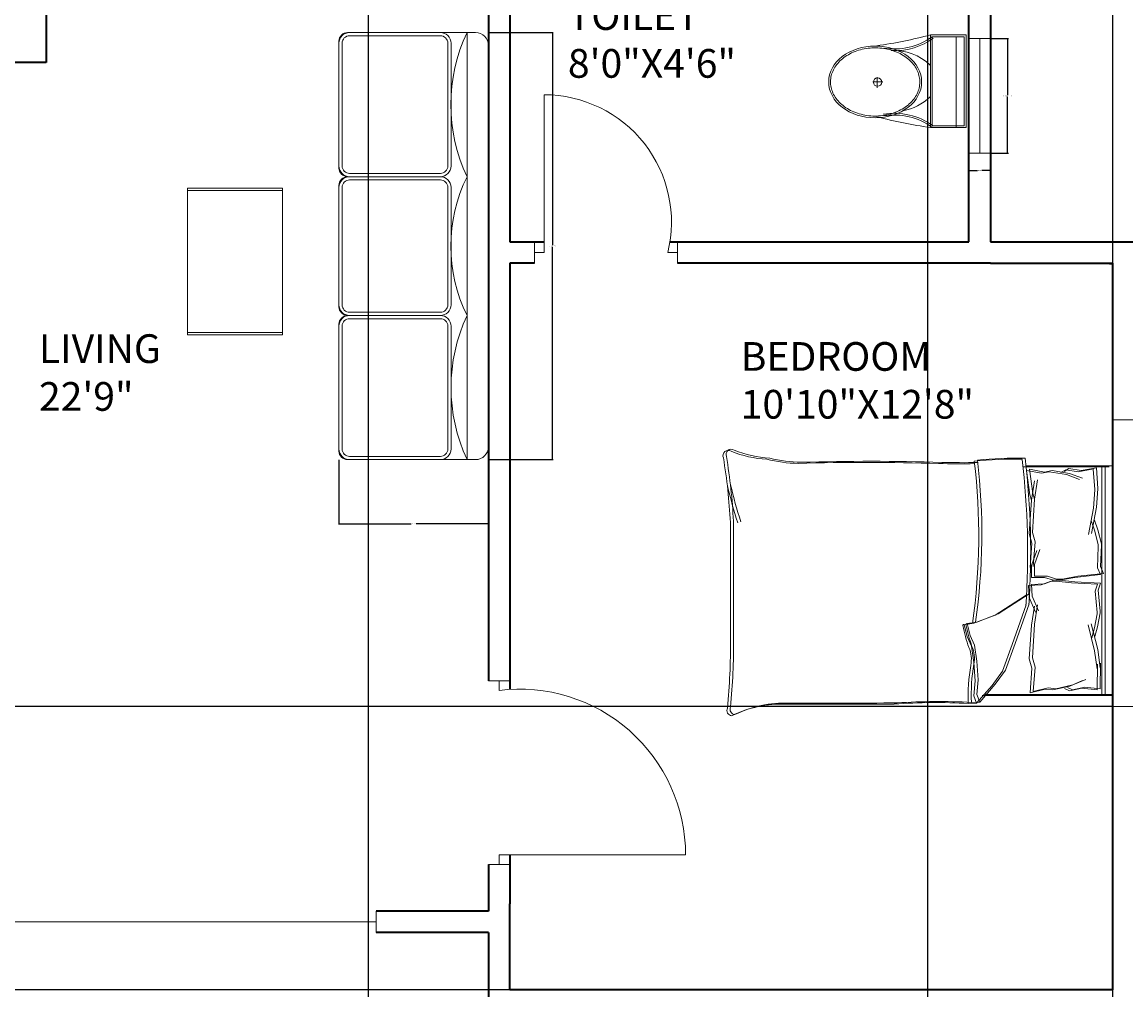
# Model space of a CAD drawing. Units: inches. Extents: x 1854 to 2495, y 1460 to 2772.
# Tile 4 of 12: x 2144 to 2375, y 1644 to 1847. Entities that reach past the tile are written whole.
import ezdxf

# ---------------------------------------------------------------- set-up
doc = ezdxf.new("R2010")
doc.units = ezdxf.units.IN
for name, color, linetype, lineweight in [('A-ANNO-DIMS', 2, 'Continuous', 18), ('A-AREA-IDEN', 7, 'Continuous', 18), ('A-DOOR', 3, 'Continuous', 18), ('A-FLOR-FIXT', 9, 'Continuous', 18), ('A-FURN', 8, 'Continuous', 13), ('A-GLAZ', 4, 'Continuous', 18), ('A-WALL', 7, 'Continuous', 35)]:
    doc.layers.add(name, color=color, linetype=linetype, lineweight=lineweight)
doc.styles.get("Standard").update_dxf_attribs({"font": 'arial.ttf'})
doc.dimstyles.get("Standard").update_dxf_attribs({"dimtxt": 0.18, "dimasz": 0.18, "dimexe": 0.18, "dimexo": 0.0625, "dimgap": 0.09, "dimtad": 0, "dimtih": 1, "dimtoh": 1, "dimdec": 4, "dimzin": 0, "dimdsep": 46, "dimtxsty": 'Standard', "dimcen": 0.09, "dimadec": 0, "dimazin": 0, "dimtfac": 1, "dimtdec": 4, "dimtofl": 0, "dimtmove": 0, "dimatfit": 3, "dimfxl": 1, "dimtolj": 1, "dimtzin": 0, "dimarcsym": 0})

# ---------------------------------------------------------------- blocks, each defined once
blk = doc.blocks.new('A$C31115884')
for p, q in [((283.1, 497.7), (223.4, 497.7)), ((257.5, 466.4), (257.5, 523.2)), ((0, 200), (0, 0)), ((520, 200), (0, 200)), ((10, 190), (10, 10)), ((510, 190), (10, 190)), ((510, 10), (510, 190)), ((520, 0), (520, 200)), ((510, 54.5), (0, 54.5)), ((10, 10), (510, 10)), ((0, 0), (520, 0))]:
    blk.add_line(p, q)
blk.add_circle((255.6, 496.4), 23.6)
for centre, radius, start, end in [((2777.7, -204.6), 2807, 165.4549, 171.71327), ((3237, 905), 2807, 188.28673, 194.5451), ((-294.5, 403.3), 364.7, 324.20913, 9.34987), ((-294.5, 403.3), 374.7, 324.20913, 9.34987), ((805.8, 403.3), 364.7, 170.65013, 215.79087), ((139.5, 406.2), 293.5, 315.84364, 2.65635), ((805.8, 403.3), 374.7, 179.20365, 215.79087), ((383.6, 406.2), 293.5, 190.27735, 224.15636)]:
    blk.add_arc(centre, radius, start, end)
blk.add_ellipse((256.2, 509.9), major_axis=(0, -260.7), ratio=0.772727)
blk.add_open_spline([(256.2, 259.2), (263.1, 259.2), (270, 259.7), (287.8, 262.3), (298.7, 265.1), (319.9, 273.1), (330.2, 278.4), (350.1, 291.1), (359.7, 298.7), (377.7, 315.9), (386.2, 325.5), (401.7, 346.6), (408.8, 358.1), (421.3, 382.5), (426.8, 395.5), (435.9, 422.4), (439.5, 436.4), (444.8, 465.1), (446.5, 479.7), (447.9, 509.2), (447.6, 524), (445, 553.3), (442.7, 567.8), (436.3, 596), (432.1, 609.7), (421.9, 636), (416, 648.6), (402.5, 672.1), (395, 683), (378.6, 703), (369.8, 712.1), (351.1, 728), (341.3, 734.8), (320.9, 746.2), (310.4, 750.7), (288.9, 757.3), (278, 759.4), (256, 761), (245, 760.6), (223.1, 757.2), (212.3, 754.3), (191.1, 746.1), (180.8, 740.7), (160.9, 727.8), (151.4, 720.1), (133.5, 702.7), (125.1, 693), (109.6, 671.7), (102.6, 660.2), (90.2, 635.7), (84.9, 622.7), (76, 595.6), (72.4, 581.6), (67.2, 552.9), (65.6, 538.2), (64.4, 508.8), (64.8, 494), (67.5, 464.7), (69.9, 450.2), (76.6, 422), (80.8, 408.3), (91.1, 382.2), (97.2, 369.7), (110.8, 346.3), (118.4, 335.4), (134.8, 315.6), (143.7, 306.7), (162.4, 290.9), (172.3, 284.2), (192.8, 273), (203.3, 268.6), (224.8, 262.2), (235.8, 260.2), (249.9, 259.3), (253, 259.2), (256.2, 259.2)], degree=3, knots=[0, 0, 0, 0, 0.110105, 0.110105, 0.285049, 0.285049, 0.459994, 0.459994, 0.634938, 0.634938, 0.809882, 0.809882, 0.984827, 0.984827, 1.159771, 1.159771, 1.334715, 1.334715, 1.50966, 1.50966, 1.684604, 1.684604, 1.859549, 1.859549, 2.034493, 2.034493, 2.209437, 2.209437, 2.384382, 2.384382, 2.559326, 2.559326, 2.73427, 2.73427, 2.909215, 2.909215, 3.084159, 3.084159, 3.259103, 3.259103, 3.434048, 3.434048, 3.608992, 3.608992, 3.783936, 3.783936, 3.958881, 3.958881, 4.133825, 4.133825, 4.30877, 4.30877, 4.483714, 4.483714, 4.658658, 4.658658, 4.833603, 4.833603, 5.008547, 5.008547, 5.183491, 5.183491, 5.358436, 5.358436, 5.53338, 5.53338, 5.708324, 5.708324, 5.883269, 5.883269, 6.058213, 6.058213, 6.233158, 6.233158, 6.283185, 6.283185, 6.283185, 6.283185])
blk = doc.blocks.new('BED-DOUBLE')
for p, q in [((30.13, 53.18), (28.39, 53.1, 3.87)), ((30.13, 53.18), (28.39, 53.1, 3.87)), ((0, 51.27), (0, 51.49)), ((0, 51.49), (0.64, 51.49)), ((0, 51.27), (26.61, 51.27)), ((0, 51.27), (26.61, 51.27)), ((0, 51.27), (0, 3.48)), ((0.64, 51.49), (27.25, 51.49)), ((0.64, 51.49), (27.25, 51.49)), ((1.53, 3.48), (1.53, 51.27)), ((1.53, 3.48), (1.53, 51.27)), ((2.17, 3.7), (2.17, 51.49)), ((2.17, 3.7), (2.17, 51.49)), ((17.21, 50.93), (14.07, 50.15)), ((17.21, 50.93), (14.07, 50.15)), ((16.81, 45.8), (17.21, 50.93)), ((16.81, 45.79), (17.21, 50.93)), ((27.75, 52.87), (24.5, 49.16)), ((27.75, 52.87), (24.5, 49.16)), ((28.39, 53.1), (25.14, 49.39)), ((28.39, 53.1), (25.14, 49.39)), ((29.49, 52.95), (27.75, 52.87, 3.87)), ((29.49, 52.95), (27.75, 52.87, 3.87)), ((28.37, 51.33), (27.75, 52.87)), ((28.37, 51.33), (27.75, 52.87)), ((28.06, 48.23), (28.37, 51.33)), ((28.06, 48.23), (28.37, 51.33)), ((29, 51.56), (28.39, 53.1)), ((29, 51.56), (28.39, 53.1)), ((28.7, 48.46), (29, 51.56)), ((28.7, 48.46), (29, 51.56)), ((2.56, 50.11), (2.46, 44.71)), ((2.56, 50.11), (2.46, 44.71)), ((2.56, 50.11), (5.77, 49.73)), ((2.56, 50.11), (5.77, 49.73)), ((3.2, 50.34), (3.1, 44.94)), ((3.2, 50.34), (3.1, 44.94)), ((3.2, 50.34), (6.41, 49.96)), ((3.2, 50.34), (6.41, 49.96)), ((8.26, 49.31), (5.58, 48.13)), ((8.26, 49.31), (5.58, 48.13)), ((5.77, 49.73), (8.34, 50.33)), ((5.77, 49.73), (8.34, 50.33)), ((8.9, 49.54), (6.22, 48.36)), ((8.9, 49.54), (6.22, 48.36)), ((6.41, 49.96), (8.98, 50.56)), ((6.41, 49.96), (8.98, 50.56)), ((11.83, 50.11), (8.26, 49.31)), ((11.83, 50.11), (8.26, 49.31)), ((8.34, 50.33), (9.38, 49.81)), ((8.34, 50.33), (9.38, 49.81)), ((12.47, 50.34), (8.9, 49.54)), ((12.47, 50.34), (8.9, 49.54)), ((8.98, 50.56), (10.02, 50.04)), ((8.98, 50.56), (10.02, 50.04)), ((13.43, 49.92), (11.83, 50.11)), ((13.43, 49.92), (11.83, 50.11)), ((14.07, 50.15), (12.47, 50.34)), ((14.07, 50.15), (12.47, 50.34)), ((16.57, 50.7), (13.43, 49.92)), ((16.57, 50.7), (13.43, 49.92)), ((16.17, 45.57), (16.57, 50.7)), ((16.17, 45.57), (16.57, 50.7)), ((24.5, 49.16), (22.33, 46.22)), ((24.5, 49.16), (22.33, 46.22)), ((25.14, 49.39), (22.97, 46.45)), ((25.14, 49.39), (22.97, 46.45)), ((22.33, 46.22), (20.32, 40.64)), ((22.33, 46.22), (20.32, 40.64)), ((22.97, 46.45), (20.96, 40.87)), ((22.97, 46.45), (20.96, 40.87)), ((28.37, 44.36), (28.06, 48.23)), ((28.37, 44.36), (28.06, 48.23)), ((29, 44.59), (28.7, 48.46)), ((29, 44.59), (28.7, 48.46)), ((2.46, 44.71), (2.54, 45.71)), ((2.46, 44.71), (2.54, 45.71)), ((2.54, 45.71), (3.07, 41.91)), ((2.54, 45.71), (3.07, 41.91)), ((3.1, 44.94), (3.18, 45.94)), ((3.1, 44.94), (3.18, 45.94)), ((3.18, 45.94), (3.71, 42.14)), ((3.18, 45.94), (3.71, 42.14)), ((16.73, 43.61), (16.17, 45.57)), ((16.73, 43.61), (16.17, 45.57)), ((17.37, 43.83), (16.81, 45.8)), ((17.37, 43.83), (16.81, 45.79)), ((28.83, 40.95), (28.37, 44.36)), ((28.83, 40.95), (28.37, 44.36)), ((29.47, 41.18), (29, 44.59)), ((29.47, 41.18), (29, 44.59)), ((3.07, 41.91), (4.42, 36.5)), ((3.07, 41.91), (4.42, 36.5)), ((3.71, 42.14), (5.06, 36.72)), ((3.71, 42.14), (5.06, 36.72)), ((16.3, 36.6), (16.73, 43.61)), ((16.3, 36.6), (16.73, 43.61)), ((16.93, 36.82), (17.37, 43.83)), ((16.93, 36.82), (17.37, 43.83)), ((4.31, 39.43), (3.72, 37.36)), ((4.31, 39.43), (3.72, 37.36)), ((20.32, 40.64), (17.38, 32.31)), ((20.32, 40.64), (17.38, 32.31)), ((20.96, 40.87), (18.02, 32.53)), ((20.96, 40.87), (18.02, 32.53)), ((29.76, 38.94), (28.83, 40.95)), ((29.76, 38.94), (28.83, 40.95)), ((30.4, 39.17), (29.47, 41.18)), ((30.4, 39.17), (29.47, 41.18)), ((79.25, 15.06), (79.25, 39.68)), ((79.25, 15.06), (79.25, 39.68)), ((79.88, 15.29), (79.88, 39.91)), ((79.88, 15.29), (79.88, 39.91)), ((3.08, 37.14), (2.54, 34.2)), ((3.08, 37.14), (2.54, 34.2)), ((3.67, 39.2), (3.08, 37.14)), ((3.67, 39.2), (3.08, 37.14)), ((3.72, 37.36), (3.18, 34.43)), ((3.72, 37.36), (3.18, 34.43)), ((30.38, 36.46), (29.76, 38.94)), ((30.38, 36.46), (29.76, 38.94)), ((31.02, 36.69), (30.4, 39.17)), ((31.02, 36.69), (30.4, 39.17)), ((15.63, 32.56), (16.3, 36.6)), ((15.63, 32.56), (16.3, 36.6)), ((16.27, 32.79), (16.93, 36.82)), ((16.27, 32.79), (16.93, 36.82)), ((18.02, 30.49), (24.52, 34.68)), ((18.02, 30.49), (24.52, 34.68)), ((23.88, 34.45), (28.37, 36.15)), ((23.88, 34.45), (28.37, 36.15)), ((24.52, 34.68), (29, 36.38)), ((24.52, 34.68), (29, 36.38)), ((28.37, 36.15), (30.38, 36.46)), ((28.37, 36.15), (30.38, 36.46)), ((29, 36.38), (31.02, 36.69)), ((29, 36.38), (31.02, 36.69)), ((2.54, 34.2), (2.56, 33.88)), ((2.54, 34.2), (2.56, 33.88)), ((2.56, 33.88), (2.98, 29.46)), ((2.56, 33.88), (2.98, 29.46)), ((3.18, 34.43), (3.2, 34.11)), ((3.18, 34.43), (3.2, 34.11)), ((3.2, 34.11), (3.62, 29.68)), ((3.2, 34.11), (3.62, 29.68)), ((16.74, 30.75), (15.45, 33.82)), ((16.74, 30.75), (15.45, 33.82)), ((17.38, 30.98), (16.09, 34.05)), ((17.38, 30.98), (16.09, 34.05)), ((17.38, 30.26), (23.88, 34.45)), ((17.38, 30.26), (23.88, 34.45)), ((16.89, 28.3), (16.74, 30.75)), ((16.89, 28.3), (16.74, 30.75)), ((17.53, 28.53), (17.38, 30.98)), ((17.53, 28.53), (17.38, 30.98)), ((2.98, 29.46), (2.49, 27.98)), ((2.98, 29.46), (2.49, 27.98)), ((2.49, 27.98), (7.87, 27.73)), ((2.49, 27.98), (7.87, 27.73)), ((3.62, 29.68), (3.13, 28.21)), ((3.62, 29.68), (3.13, 28.21)), ((3.13, 28.21), (8.51, 27.96)), ((3.13, 28.21), (8.51, 27.96)), ((7.87, 27.73), (11.08, 27.36)), ((7.87, 27.73), (11.08, 27.35)), ((8.51, 27.96), (11.72, 27.58)), ((8.51, 27.96), (11.72, 27.58)), ((12.38, 27.44), (14.22, 28.13)), ((12.38, 27.44), (14.22, 28.13)), ((13.02, 27.66), (14.86, 28.36)), ((13.02, 27.66), (14.86, 28.36)), ((14.22, 28.13), (16.89, 28.3)), ((14.22, 28.13), (16.89, 28.3)), ((14.86, 28.36), (17.53, 28.53)), ((14.86, 28.36), (17.53, 28.53)), ((1.87, 25.98), (7.22, 26.56)), ((1.87, 25.98), (7.22, 26.56)), ((2.45, 24.54), (1.87, 25.98)), ((2.45, 24.54), (1.87, 25.98)), ((2.51, 26.21), (7.86, 26.79)), ((2.51, 26.21), (7.86, 26.79)), ((3.09, 24.77), (2.51, 26.21)), ((3.09, 24.77), (2.51, 26.21)), ((7.22, 26.56), (10.4, 27.14)), ((7.22, 26.56), (10.4, 27.14)), ((7.86, 26.79), (11.04, 27.37)), ((7.86, 26.79), (11.04, 27.37)), ((10.4, 27.14), (11.7, 27.14)), ((10.4, 27.14), (11.7, 27.14)), ((11.04, 27.37), (12.34, 27.37)), ((11.04, 27.37), (12.34, 27.37)), ((11.08, 27.36), (12.38, 27.44)), ((11.08, 27.35), (12.38, 27.44)), ((11.7, 27.14), (13.58, 26.56)), ((11.7, 27.14), (13.58, 26.56)), ((11.72, 27.58), (13.02, 27.66)), ((11.72, 27.58), (13.02, 27.66)), ((12.34, 27.37), (14.22, 26.79)), ((12.34, 27.37), (14.22, 26.79)), ((13.58, 26.56), (16.26, 26.56)), ((13.58, 26.56), (16.26, 26.56)), ((14.22, 26.79), (16.9, 26.79)), ((14.22, 26.79), (16.9, 26.79)), ((16.26, 26.56), (16.26, 24.1)), ((16.26, 26.56), (16.26, 24.1)), ((16.9, 26.79), (16.9, 24.33)), ((16.9, 26.79), (16.9, 24.33)), ((2.3, 20.09), (2.45, 24.54)), ((2.3, 20.09), (2.45, 24.54)), ((2.94, 20.32), (3.09, 24.77)), ((2.94, 20.32), (3.09, 24.77)), ((16.26, 24.1), (15.17, 20.96)), ((16.26, 24.1), (15.17, 20.96)), ((16.9, 24.33), (15.81, 21.19)), ((16.9, 24.33), (15.81, 21.19)), ((16.17, 19.38), (16.57, 24.52)), ((16.17, 19.38), (16.57, 24.52)), ((16.81, 19.61), (17.21, 24.74)), ((16.81, 19.61), (17.21, 24.74)), ((2.3, 19.77), (2.3, 20.09)), ((2.3, 19.77), (2.3, 20.09)), ((3.03, 16.88), (2.3, 19.77)), ((3.03, 16.88), (2.3, 19.77)), ((2.94, 20), (2.94, 20.32)), ((2.94, 20), (2.94, 20.32)), ((3.67, 17.11), (2.94, 20)), ((3.67, 17.11), (2.94, 20)), ((16.73, 17.42), (16.17, 19.38)), ((16.73, 17.42), (16.17, 19.38)), ((17.37, 17.65), (16.81, 19.61)), ((17.37, 17.65), (16.81, 19.61)), ((3.75, 14.86), (3.03, 16.88)), ((3.75, 14.85), (3.03, 16.88)), ((3.32, 12.11), (4.33, 17.6)), ((3.32, 12.11), (4.33, 17.6)), ((4.39, 15.08), (3.67, 17.11)), ((4.39, 15.08), (3.67, 17.11)), ((3.96, 12.34), (4.97, 17.83)), ((3.96, 12.34), (4.97, 17.83)), ((16.3, 10.41), (16.73, 17.42)), ((16.3, 10.41), (16.73, 17.42)), ((16.93, 10.64), (17.37, 17.65)), ((16.93, 10.64), (17.37, 17.65)), ((3.03, 8.29), (3.32, 12.11)), ((3.03, 8.28), (3.32, 12.11)), ((3.67, 8.51), (3.96, 12.34)), ((3.67, 8.51), (3.96, 12.34)), ((15.63, 6.38), (16.3, 10.41)), ((15.63, 6.38), (16.3, 10.41)), ((16.27, 6.61), (16.93, 10.64)), ((16.27, 6.61), (16.93, 10.64)), ((16.3, 10.41), (16.62, 9.28)), ((16.3, 10.41), (16.62, 9.28)), ((16.62, 9.28), (17.34, 4.18)), ((16.62, 9.28), (17.34, 4.18)), ((16.93, 10.64), (17.26, 9.51)), ((16.93, 10.64), (17.26, 9.51)), ((17.26, 9.51), (17.98, 4.41)), ((17.26, 9.51), (17.98, 4.41)), ((3.01, 8.18), (3.03, 8.29)), ((3.01, 8.18), (3.03, 8.28)), ((3.34, 3.9), (3.01, 8.18)), ((3.34, 3.9), (3.01, 8.18)), ((3.65, 8.41), (3.67, 8.51)), ((3.65, 8.41), (3.67, 8.51)), ((3.98, 4.13), (3.65, 8.41)), ((3.98, 4.13), (3.65, 8.41)), ((3.96, 4.12), (7.14, 4.7)), ((3.96, 4.12), (7.14, 4.7)), ((8.96, 5.05), (6.21, 6.06)), ((8.96, 5.05), (6.21, 6.06)), ((9.59, 5.28), (6.85, 6.29)), ((9.59, 5.28), (6.85, 6.29)), ((7.14, 4.7), (9.74, 4.27)), ((7.14, 4.7), (9.74, 4.27)), ((12.57, 4.47), (8.96, 5.05)), ((12.57, 4.47), (8.96, 5.05)), ((9.1, 4.04), (10.11, 4.62)), ((13.21, 4.7), (9.59, 5.28)), ((13.21, 4.7), (9.59, 5.28)), ((9.74, 4.27), (10.75, 4.85)), ((9.74, 4.27), (10.75, 4.85)), ((14.16, 4.76), (12.57, 4.47)), ((14.16, 4.76), (12.57, 4.47)), ((14.8, 4.99), (13.21, 4.7)), ((14.8, 4.99), (13.21, 4.7)), ((17.34, 4.18), (14.16, 4.76)), ((17.34, 4.18), (14.16, 4.76)), ((17.98, 4.41), (14.8, 4.99)), ((17.98, 4.41), (14.8, 4.99)), ((18.11, 3.48), (0, 3.48)), ((18.11, 3.48), (0, 3.48)), ((18.75, 3.7), (0.64, 3.7)), ((18.75, 3.7), (0.64, 3.7)), ((3.32, 3.89), (6.5, 4.47)), ((3.32, 3.89), (6.5, 4.47)), ((6.5, 4.47), (9.1, 4.04)), ((6.5, 4.47), (9.1, 4.04)), ((9.1, 4.04), (10.11, 4.62))]:
    blk.add_line(p, q)
for centre, radius, start, end in [((68.67, 76.16), 23.07, 267.4714, 296.4681), ((68.67, 76.16), 23.07, 267.4714, 296.4681), ((69.31, 76.39), 23.07, 267.4714, 296.4681), ((69.31, 76.39), 23.07, 267.4714, 296.4681), ((78.87, 54.41), 1.1, 332.6588, 86.02), ((78.87, 54.41), 1.1, 332.6588, 86.02), ((79.51, 54.64), 1.1, 332.6588, 86.02), ((79.51, 54.64), 1.1, 332.6588, 86.02), ((-6.02, 51.56), 36.18, 349.8763, 2.5657), ((-6.02, 51.56), 36.18, 349.8763, 2.5657), ((36.95, 182.49), 129.5, 266.9791, 273.8365), ((36.95, 182.49), 129.5, 266.9791, 273.8365), ((67.82, -4508.74), 4561.86, 90.00217, 90.28689), ((67.82, -4508.74), 4561.86, 90.00217, 90.28689), ((68.46, -4508.51), 4561.86, 90.00217, 90.28689), ((68.46, -4508.52), 4561.86, 90.00217, 90.28689), ((212.28, 41.15), 133.04, 174.4998, 180.6351), ((212.28, 41.15), 133.04, 174.4998, 180.6351), ((212.92, 41.38), 133.04, 174.4998, 180.6351), ((212.92, 41.38), 133.04, 174.4998, 180.6351), ((-6.66, 51.33), 36.18, 349.8763, 2.5657), ((-6.66, 51.33), 36.18, 349.8763, 2.5657), ((36.32, 182.27), 129.5, 266.9791, 273.8365), ((36.32, 182.27), 129.5, 266.9791, 273.8365), ((35.07, 43.74), 6.22, 168.6608, 203.7384), ((35.07, 43.74), 6.22, 168.6608, 203.7384), ((35.71, 43.97), 6.22, 168.6608, 203.7384), ((35.71, 43.97), 6.22, 168.6608, 203.7384), ((1.48, 31.15), 29.65, 10.6617, 19.8806), ((1.48, 31.15), 29.65, 10.6617, 19.8806), ((2.12, 31.38), 29.65, 10.6617, 19.8806), ((2.12, 31.38), 29.65, 10.6617, 19.8806), ((156.32, 17.76), 129.02, 171.7845, 186.9006), ((156.32, 17.76), 129.02, 171.7845, 186.9006), ((156.96, 17.98), 129.02, 171.7845, 186.9006), ((156.96, 17.98), 129.02, 171.7845, 186.9006), ((30.44, 36.64), 0.185, 250.2464, 1.1377), ((30.44, 36.64), 0.185, 250.2464, 1.1377), ((31.08, 36.86), 0.185, 250.2464, 1.1377), ((31.08, 36.86), 0.185, 250.2464, 1.1377), ((182.05, 21.36), 164.97, 176.0865, 186.7821), ((182.05, 21.36), 164.97, 176.0865, 186.7821), ((182.69, 21.59), 164.97, 176.0865, 186.7821), ((182.69, 21.59), 164.97, 176.0865, 186.7821), ((-23.71, -17.22), 106.46, 13.3832, 17.7053), ((-23.71, -17.22), 106.46, 13.3832, 17.7053), ((-23.07, -16.99), 106.46, 13.3832, 17.7053), ((-23.07, -16.99), 106.46, 13.3832, 17.7053), ((200.84, 21.43), 121.76, 182.9958, 189.4091), ((200.84, 21.43), 121.76, 182.9958, 189.4091), ((201.48, 21.66), 121.76, 182.9958, 189.4091), ((201.48, 21.66), 121.76, 182.9958, 189.4091), ((20.74, 85.39), 83.31, 268.7218, 275.604), ((20.74, 85.39), 83.31, 268.7218, 275.604), ((31.17, -167.31), 170.11, 88.4762, 91.0082), ((31.17, -167.31), 170.11, 88.4762, 91.0082), ((31.81, -167.08), 170.11, 88.4762, 91.0082), ((31.81, -167.08), 170.11, 88.4762, 91.0082), ((50.61, 484.82), 482.31, 268.2277, 271.7185), ((50.61, 484.82), 482.31, 268.2277, 271.7185), ((51.25, 485.05), 482.31, 268.2277, 271.7185), ((51.25, 485.05), 482.31, 268.2277, 271.7185), ((64.52, -26.9), 29.63, 76.0648, 88.9113), ((64.52, -26.9), 29.63, 76.0648, 88.9113), ((65.15, -26.67), 29.63, 76.0648, 88.9113), ((65.15, -26.67), 29.63, 76.0648, 88.9113), ((20.1, 85.16), 83.31, 268.7218, 275.604), ((20.1, 85.16), 83.31, 268.7218, 275.604), ((70.28, -21.66), 23.56, 67.9751, 86.652), ((70.28, -21.66), 23.56, 67.9751, 86.652), ((70.92, -21.43), 23.56, 67.9751, 86.652), ((70.92, -21.43), 23.56, 67.9751, 86.652), ((79.72, 1.09), 1.09, 236.1736, 23.4781), ((79.72, 1.09), 1.09, 236.1736, 23.4781), ((80.36, 1.32), 1.09, 236.1736, 23.4781), ((80.36, 1.32), 1.09, 236.1736, 23.4781)]:
    blk.add_arc(centre, radius, start, end)
blk = doc.blocks.new('TABLE-COFFEE')
blk.add_lwpolyline([(0, 30.16), (19.85, 30.16), (19.85, 0), (0, 0)], close=True)
blk = doc.blocks.new('WINDOW-60IN')
for p, q in [((0, 9), (0, 0)), ((60, 4.5), (60, 9)), ((60, 9), (60, 0)), ((0, 0), (0, 4.5)), ((0, 4.5), (60, 4.5))]:
    blk.add_line(p, q)
blk = doc.blocks.new('DOOR-39IN-SWING')
blk.add_line((39, 0), (0, 0))
blk.add_arc((34.67, 0), 34.66, 82.8159, 180)
blk = doc.blocks.new('WINDOW-VENT-24IN-INTERIOR')
for p, q in [((0, 24), (4.5, 24)), ((2.25, 24), (2.25, 0)), ((0, 0), (4.5, 0))]:
    blk.add_line(p, q)
blk = doc.blocks.new('SOFA-3-SEAT')
for points in [[(2.23, 59.19), (21.22, 59.19, 0.414214), (23.45, 61.43), (23.45, 87.12, 0.414214), (21.22, 89.35), (2.23, 89.35, 0.414214), (0, 87.12), (0, 61.43, 0.414214)], [(2.23, 59.19), (21.22, 59.19, -0.414214), (23.45, 56.96), (23.45, 32.39, -0.414214), (21.22, 30.16), (2.23, 30.16, -0.414214), (0, 32.39), (0, 56.96, -0.414214)], [(2.23, 0), (21.22, 0, 0.414214), (23.45, 2.23), (23.45, 27.92, 0.414214), (21.22, 30.16), (2.23, 30.16, 0.414214), (0, 27.92), (0, 2.23, 0.414214)]]:
    blk.add_lwpolyline(points, format="xyb", close=True)
at = {"ltscale": 0.03}
blk.add_lwpolyline([(0, 28.35), (0, 1.79, 0.414214), (1.79, 0), (28.59, 0, 0.414214), (31.27, 2.68), (31.27, 86.67, 0.414214), (28.59, 89.35), (1.79, 89.35, 0.414214), (0, 87.56), (0, 61, 0.414214), (1.79, 59.22, -1), (1.79, 59.17, 0.414214), (0, 57.38), (0, 31.96, 0.414214), (1.79, 30.18, -1), (1.79, 30.13, 0.414214)], format="xyb", close=True, dxfattribs=at)
blk.add_lwpolyline([(26.8, 0), (26.8, 89.35)])
for centre, radius, start, end in [((58.64, 74.27), 35.22, 154.6538, 205.3462), ((56.4, 44.67), 32.97, 153.869, 206.131), ((59.01, 15.08), 35.56, 154.9106, 205.0894)]:
    blk.add_arc(centre, radius, start, end)
blk = doc.blocks.new('*D37')
at = {"layer": 'A-ANNO-DIMS', "color": 0, "lineweight": -2, "transparency": 16777216}
for p, q in [((2346.54, 1843.06), (2350.26, 1843.06)), ((2350.08, 1842.88), (2350.08, 1831.24)), ((2350.08, 1819.24), (2350.08, 1830.88)), ((2346.54, 1819.06), (2350.26, 1819.06))]:
    blk.add_line(p, q, dxfattribs=at)
at = {"layer": 'A-ANNO-DIMS', "color": 0, "transparency": 16777216}
for points in [[(2350.05, 1842.88), (2350.11, 1842.88), (2350.08, 1843.06)], [(2350.05, 1819.24), (2350.11, 1819.24), (2350.08, 1819.06)]]:
    blk.add_solid(points, dxfattribs=at)
at = {"layer": 'Defpoints', "color": 0, "transparency": 16777216}
for p in [(2346.48, 1843.06), (2350.08, 1843.06), (2346.48, 1819.06)]:
    blk.add_point(p, dxfattribs=at)
at = {"layer": 'A-ANNO-DIMS', "color": 0, "transparency": 16777216, "insert": (2350.08, 1831.06), "char_height": 0.18, "attachment_point": 5}
blk.add_mtext('\\A1;INT. VENT 24 TYP.', dxfattribs=at)
blk = doc.blocks.new('*D38')
at = {"layer": 'A-ANNO-DIMS', "color": 0, "lineweight": -2, "transparency": 16777216}
for p, q in [((2341.98, 1819), (2341.98, 1815.28)), ((2346.48, 1819), (2346.48, 1815.28)), ((2342.16, 1815.46), (2343.77, 1815.46)), ((2346.3, 1815.46), (2344.69, 1815.46))]:
    blk.add_line(p, q, dxfattribs=at)
at = {"layer": 'A-ANNO-DIMS', "color": 0, "transparency": 16777216}
for points in [[(2342.16, 1815.49), (2342.16, 1815.43), (2341.98, 1815.46)], [(2346.3, 1815.49), (2346.3, 1815.43), (2346.48, 1815.46)]]:
    blk.add_solid(points, dxfattribs=at)
at = {"layer": 'Defpoints', "color": 0, "transparency": 16777216}
for p in [(2341.98, 1819.06), (2346.48, 1819.06), (2346.48, 1815.46)]:
    blk.add_point(p, dxfattribs=at)
at = {"layer": 'A-ANNO-DIMS', "color": 0, "transparency": 16777216, "insert": (2344.23, 1815.46), "char_height": 0.18, "attachment_point": 5}
blk.add_mtext('\\A1;5 TYP.', dxfattribs=at)
blk = doc.blocks.new('*D47')
at = {"layer": 'A-ANNO-DIMS', "color": 0, "lineweight": -2, "transparency": 16777216}
for p, q in [((2241.54, 1844.33), (2255.06, 1844.33)), ((2254.88, 1844.15), (2254.88, 1799.84)), ((2254.88, 1755.16), (2254.88, 1799.47)), ((2241.54, 1754.98), (2255.06, 1754.98))]:
    blk.add_line(p, q, dxfattribs=at)
at = {"layer": 'A-ANNO-DIMS', "color": 0, "transparency": 16777216}
for points in [[(2254.85, 1844.15), (2254.91, 1844.15), (2254.88, 1844.33)], [(2254.85, 1755.16), (2254.91, 1755.16), (2254.88, 1754.98)]]:
    blk.add_solid(points, dxfattribs=at)
at = {"layer": 'Defpoints', "color": 0, "transparency": 16777216}
for p in [(2241.48, 1844.33), (2254.88, 1844.33), (2241.48, 1754.98)]:
    blk.add_point(p, dxfattribs=at)
at = {"layer": 'A-ANNO-DIMS', "color": 0, "transparency": 16777216, "insert": (2254.88, 1799.66), "char_height": 0.18, "attachment_point": 5}
blk.add_mtext('\\A1;SOFA 89 TYP.', dxfattribs=at)
blk = doc.blocks.new('*D48')
at = {"layer": 'A-ANNO-DIMS', "color": 0, "lineweight": -2, "transparency": 16777216}
for p, q in [((2210.21, 1754.92), (2210.21, 1741.4)), ((2241.48, 1754.92), (2241.48, 1741.4)), ((2210.39, 1741.58), (2225.32, 1741.58)), ((2241.3, 1741.58), (2226.37, 1741.58))]:
    blk.add_line(p, q, dxfattribs=at)
at = {"layer": 'A-ANNO-DIMS', "color": 0, "transparency": 16777216}
for points in [[(2210.39, 1741.61), (2210.39, 1741.55), (2210.21, 1741.58)], [(2241.3, 1741.61), (2241.3, 1741.55), (2241.48, 1741.58)]]:
    blk.add_solid(points, dxfattribs=at)
at = {"layer": 'Defpoints', "color": 0, "transparency": 16777216}
for p in [(2210.21, 1754.98), (2241.48, 1754.98), (2241.48, 1741.58)]:
    blk.add_point(p, dxfattribs=at)
at = {"layer": 'A-ANNO-DIMS', "color": 0, "transparency": 16777216, "insert": (2225.85, 1741.58), "char_height": 0.18, "attachment_point": 5}
blk.add_mtext('\\A1;31 TYP.', dxfattribs=at)
blk = doc.blocks.new('*D50')
at = {"layer": 'A-ANNO-DIMS', "color": 0, "lineweight": -2, "transparency": 16777216}
for p, q in [((2381.04, 2272.04), (2418.21, 2272.04)), ((2418.03, 2271.86), (2418.03, 1933.48)), ((2418.03, 1594.72), (2418.03, 1933.11)), ((2119.04, 1594.54), (2418.21, 1594.54))]:
    blk.add_line(p, q, dxfattribs=at)
at = {"layer": 'A-ANNO-DIMS', "color": 0, "transparency": 16777216}
for points in [[(2418, 2271.86), (2418.06, 2271.86), (2418.03, 2272.04)], [(2418, 1594.72), (2418.06, 1594.72), (2418.03, 1594.54)]]:
    blk.add_solid(points, dxfattribs=at)
at = {"layer": 'Defpoints', "color": 0, "transparency": 16777216}
for p in [(2380.98, 2272.04), (2418.03, 2272.04), (2118.98, 1594.54)]:
    blk.add_point(p, dxfattribs=at)
at = {"layer": 'A-ANNO-DIMS', "color": 0, "transparency": 16777216, "insert": (2418.03, 1933.29), "char_height": 0.18, "attachment_point": 5}
blk.add_mtext('\\A1;677.5', dxfattribs=at)
blk = doc.blocks.new('*D64')
at = {"layer": 'A-ANNO-DIMS', "color": 0, "lineweight": -2, "transparency": 16777216}
for p, q in [((2333.32, 2262.98), (2333.32, 1503.44)), ((2371.98, 2262.98), (2371.98, 1503.44)), ((2333.5, 1503.62), (2352.26, 1503.62)), ((2371.8, 1503.62), (2353.05, 1503.62))]:
    blk.add_line(p, q, dxfattribs=at)
at = {"layer": 'A-ANNO-DIMS', "color": 0, "transparency": 16777216}
for points in [[(2333.5, 1503.65), (2333.5, 1503.59), (2333.32, 1503.62)], [(2371.8, 1503.65), (2371.8, 1503.59), (2371.98, 1503.62)]]:
    blk.add_solid(points, dxfattribs=at)
at = {"layer": 'Defpoints', "color": 0, "transparency": 16777216}
for p in [(2333.32, 2263.04), (2371.98, 2263.04), (2371.98, 1503.62)]:
    blk.add_point(p, dxfattribs=at)
at = {"layer": 'A-ANNO-DIMS', "color": 0, "transparency": 16777216, "insert": (2352.65, 1503.62), "char_height": 0.18, "attachment_point": 5}
blk.add_mtext('\\A1;38.66', dxfattribs=at)
blk = doc.blocks.new('*D66')
at = {"layer": 'A-ANNO-DIMS', "color": 0, "lineweight": -2, "transparency": 16777216}
for p, q in [((2371.92, 1703.31), (1940.75, 1703.31)), ((1940.93, 1703.13), (1940.93, 1673.86)), ((1940.93, 1644.22), (1940.93, 1673.5)), ((2371.92, 1644.04), (1940.75, 1644.04))]:
    blk.add_line(p, q, dxfattribs=at)
at = {"layer": 'A-ANNO-DIMS', "color": 0, "transparency": 16777216}
for points in [[(1940.9, 1703.13), (1940.96, 1703.13), (1940.93, 1703.31)], [(1940.9, 1644.22), (1940.96, 1644.22), (1940.93, 1644.04)]]:
    blk.add_solid(points, dxfattribs=at)
at = {"layer": 'Defpoints', "color": 0, "transparency": 16777216}
for p in [(1940.93, 1703.31), (2371.98, 1703.31), (2371.98, 1644.04)]:
    blk.add_point(p, dxfattribs=at)
at = {"layer": 'A-ANNO-DIMS', "color": 0, "transparency": 16777216, "insert": (1940.93, 1673.68), "char_height": 0.18, "attachment_point": 5}
blk.add_mtext('\\A1;59.27', dxfattribs=at)
blk = doc.blocks.new('*D73')
at = {"layer": 'A-ANNO-DIMS', "color": 0, "lineweight": -2, "transparency": 16777216}
for p, q in [((2131.08, 2220.98), (2131.08, 1503.44)), ((2216.32, 2220.98), (2216.32, 1503.44)), ((2131.26, 1503.62), (2173.31, 1503.62)), ((2216.14, 1503.62), (2174.1, 1503.62))]:
    blk.add_line(p, q, dxfattribs=at)
at = {"layer": 'A-ANNO-DIMS', "color": 0, "transparency": 16777216}
for points in [[(2131.26, 1503.65), (2131.26, 1503.59), (2131.08, 1503.62)], [(2216.14, 1503.65), (2216.14, 1503.59), (2216.32, 1503.62)]]:
    blk.add_solid(points, dxfattribs=at)
at = {"layer": 'Defpoints', "color": 0, "transparency": 16777216}
for p in [(2131.08, 2221.04), (2216.32, 2221.04), (2216.32, 1503.62)]:
    blk.add_point(p, dxfattribs=at)
at = {"layer": 'A-ANNO-DIMS', "color": 0, "transparency": 16777216, "insert": (2173.7, 1503.62), "char_height": 0.18, "attachment_point": 5}
blk.add_mtext('\\A1;85.25', dxfattribs=at)

msp = doc.modelspace()

# ---------------------------------------------------------------- linework, layer by layer
at = {"layer": 'A-DOOR'}
for p, q in [((2253.1289, 1798.3071), (2253.1289, 1831.3071)), ((2251.1289, 1800.5571), (2251.1289, 1796.0571)), ((2281.0007, 1800.5571), (2281.0007, 1796.0571)), ((2251.1289, 1796.0571), (2251.1289, 1798.3071)), ((2251.1289, 1798.3071), (2253.1289, 1798.3071)), ((2281.0007, 1798.3071), (2279.0007, 1798.3071)), ((2281.0007, 1796.0571), (2281.0007, 1798.3071)), ((2241.4824, 1708.6844), (2245.9824, 1708.6844)), ((2245.9824, 1708.6844), (2243.7324, 1708.6844)), ((2243.7324, 1708.6844), (2243.7324, 1706.6844)), ((2243.7324, 1670.2917), (2243.7324, 1672.2917)), ((2241.4824, 1670.2917), (2245.9824, 1670.2917)), ((2245.9824, 1670.2917), (2243.7324, 1670.2917))]:
    msp.add_line(p, q, dxfattribs=at)
msp.add_arc((2253.1289, 1804.6655), 26.6417, 346.192433, 90, dxfattribs=at)
at = {"layer": 'A-FURN'}
for points in [[(2212.444, 1814.8445), (2231.4306, 1814.8445, 0.41421356), (2232.9942, 1816.4081), (2232.9942, 1842.0959, 0.41421356), (2231.4306, 1843.6595), (2212.444, 1843.6595, 0.41421356), (2210.8804, 1842.0959), (2210.8804, 1816.4081, 0.41421356)], [(2212.444, 1813.5042), (2231.4306, 1813.5042, -0.41421356), (2232.9942, 1811.9406), (2232.9942, 1787.3696, -0.41421356), (2231.4306, 1785.806), (2212.444, 1785.806, -0.41421356), (2210.8804, 1787.3696), (2210.8804, 1811.9406, -0.41421356)], [(2212.444, 1755.6507), (2231.4306, 1755.6507, 0.41421356), (2232.9942, 1757.2143), (2232.9942, 1782.9022, 0.41421356), (2231.4306, 1784.4658), (2212.444, 1784.4658, 0.41421356), (2210.8804, 1782.9022), (2210.8804, 1757.2143, 0.41421356)]]:
    msp.add_lwpolyline(points, format="xyb", close=True, dxfattribs=at)
at = {"layer": 'A-GLAZ'}
for p, q in [((2346.4824, 1843.0598), (2344.2324, 1843.0598)), ((2344.2324, 1819.0598), (2341.9824, 1819.0598)), ((2218.0111, 1660.5449), (2218.0111, 1656.0449)), ((2218.0111, 1658.2949), (2140.0894, 1658.2949)), ((2218.0111, 1656.0449), (2218.0111, 1658.2949))]:
    msp.add_line(p, q, dxfattribs=at)
at = {"layer": 'A-WALL'}
for p, q in [((2148.9824, 1928.5287), (2148.9824, 1838.0449)), ((2241.4824, 1859.0571), (2241.4824, 1708.6844)), ((2245.9824, 1854.5571), (2245.9824, 1800.5571)), ((2245.9824, 1854.5571), (2245.9824, 1800.5571)), ((2341.9824, 1800.5571), (2341.9824, 1854.5571)), ((2346.4824, 1854.5571), (2346.4824, 1800.5571)), ((2148.9824, 1838.0449), (2139.9824, 1838.0449)), ((2245.9824, 1800.5571), (2253.1289, 1800.5571)), ((2279.4519, 1800.5571), (2341.9824, 1800.5571)), ((2346.4824, 1800.5571), (2380.9824, 1800.5571)), ((2371.9824, 1800.5571), (2371.9824, 1800.5449)), ((2371.9824, 1800.5571), (2371.9824, 1800.5449)), ((2251.1289, 1796.0571), (2245.9824, 1796.0571)), ((2245.9824, 1796.0571), (2245.9824, 1706.8938)), ((2346.4824, 1796.0571), (2281.0007, 1796.0571)), ((2346.4824, 1796.0571), (2371.9824, 1796.0571)), ((2371.391, 1796.0449), (2371.9824, 1796.0449)), ((2371.9824, 1796.0571), (2371.9824, 1662.0571)), ((2371.9824, 1796.0571), (2371.9824, 1644.0571)), ((2371.9824, 1796.0449), (2371.9824, 1644.0449)), ((2245.9824, 1672.2917), (2245.9824, 1662.0571)), ((2241.4824, 1670.2917), (2241.4824, 1662.0571)), ((2241.4824, 1660.5449), (2218.0111, 1660.5449)), ((2241.4824, 1662.0571), (2241.4824, 1660.5449)), ((2245.9824, 1644.0449), (2245.9824, 1662.0571)), ((2241.4824, 1656.0449), (2218.0111, 1656.0449)), ((2241.4824, 1656.0449), (2241.4824, 1644.0449)), ((2241.4824, 1644.0449), (2241.4824, 1635.0449)), ((2371.9824, 1644.0449), (2245.9824, 1644.0449))]:
    msp.add_line(p, q, dxfattribs=at)

# ---------------------------------------------------------------- block references
at = {"layer": 'A-DOOR', "extrusion": (0, 0, -1), "zscale": -1}
msp.add_blockref('DOOR-39IN-SWING', (-2282.7328, 1672.292), dxfattribs=at)
at = {"layer": 'A-FLOR-FIXT', "xscale": 0.0372717239612423, "yscale": 0.0372717239612423, "zscale": 0.0372717239612423, "rotation": 89.99999999999999}
msp.add_blockref('A$C31115884', (2341.3777, 1824.4469), dxfattribs=at)
at = {"layer": 'A-FURN'}
for name, p in [('SOFA-3-SEAT', (2210.21, 1754.9807)), ('TABLE-COFFEE', (2178.531, 1781.6019)), ('TABLE-COFFEE', (2178.531, 1781.118))]:
    msp.add_blockref(name, p, dxfattribs=at)
at = {"layer": 'A-FURN', "rotation": 180}
msp.add_blockref('BED-DOUBLE', (2371.9827, 1757.1468), dxfattribs=at)
at = {"layer": 'A-GLAZ'}
msp.add_blockref('WINDOW-VENT-24IN-INTERIOR', (2341.982, 1819.06), dxfattribs=at)
at = {"layer": 'A-GLAZ', "rotation": 270.000000000001}
msp.add_blockref('WINDOW-60IN', (2371.9825, 1763.3146), dxfattribs=at)

# ---------------------------------------------------------------- texts
at = {"layer": 'A-AREA-IDEN', "char_height": 6, "attachment_point": 1}
for s, width, insert in [('TOILET\\P8\'0"X4\'6"', 99.121381, (2258.1048, 1850.8764)), ('LIVING\\P22\'9"', 70.670702, (2147.4726, 1781.2001)), ('BEDROOM\\P10\'10"X12\'8"', 124.280546, (2294.2517, 1779.5673))]:
    msp.add_mtext_dynamic_manual_height_columns(s, width=width, gutter_width=12.5, heights=[0], dxfattribs=dict(at, insert=insert))

# ---------------------------------------------------------------- dimensions: what is measured, and where the dimension line sits
at = {"layer": 'A-ANNO-DIMS'}
for base, p1, p2, override, picture, middle in [((2418.0324, 2272.0449), (2118.9824, 1594.5449), (2380.9824, 2272.0449), {"dimdec": 1, "dimlfac": 1, "dimrnd": 0, "dimzin": 0, "dimdsep": 46, "dimlunit": 2}, '*D50', (2418.0324, 1933.2949)), ((1940.9324, 1703.3147), (2371.9824, 1644.0449), (2371.9824, 1703.3147), {"dimdec": 2, "dimlfac": 1, "dimrnd": 0, "dimzin": 0, "dimdsep": 46, "dimlunit": 2}, '*D66', (1940.9324, 1673.6798))]:
    dim = msp.add_linear_dim(base=base, p1=p1, p2=p2, angle=90, dimstyle='Standard', override=override, dxfattribs=at)
    dim.commit()
    dim.dimension.update_dxf_attribs({"geometry": picture, "text_midpoint": middle})
for base, p1, p2, picture, middle in [((2371.9824, 1503.6207), (2333.3214, 2263.0449), (2371.9824, 2263.0449), '*D64', (2352.6519, 1503.6207)), ((2216.3239, 1503.6207), (2131.0775, 2221.0449), (2216.3239, 2221.0449), '*D73', (2173.7007, 1503.6207))]:
    dim = msp.add_linear_dim(base=base, p1=p1, p2=p2, dimstyle='Standard', override={"dimdec": 2, "dimlfac": 1, "dimrnd": 0, "dimzin": 0, "dimdsep": 46, "dimlunit": 2}, dxfattribs=at)
    dim.commit()
    dim.dimension.update_dxf_attribs({"geometry": picture, "text_midpoint": middle})
for base, p1, p2, text, picture, middle in [((2254.8847, 1844.3296), (2241.4824, 1754.9806), (2241.4824, 1844.3296), 'SOFA <> TYP.', '*D47', (2254.8847, 1799.6551)), ((2350.0824, 1843.0598), (2346.4824, 1819.0598), (2346.4824, 1843.0598), 'INT. VENT <> TYP.', '*D37', (2350.0824, 1831.0598))]:
    dim = msp.add_linear_dim(base=base, p1=p1, p2=p2, angle=90, text=text, dimstyle='Standard', override={"dimdec": 0, "dimlfac": 1, "dimrnd": 0, "dimzin": 0, "dimdsep": 46, "dimlunit": 2}, dxfattribs=at)
    dim.commit()
    dim.dimension.update_dxf_attribs({"geometry": picture, "text_midpoint": middle})
for base, p1, p2, picture, middle in [((2346.4823891272, 1815.45976585), (2341.9823891272, 1819.05976585), (2346.4823891272, 1819.05976585), '*D38', (2344.2323891272, 1815.45976585)), ((2241.4824, 1741.5783), (2210.2102, 1754.9806), (2241.4824, 1754.9806), '*D48', (2225.8463, 1741.5783))]:
    dim = msp.add_linear_dim(base=base, p1=p1, p2=p2, text='<> TYP.', dimstyle='Standard', override={"dimdec": 0, "dimlfac": 1, "dimrnd": 0, "dimzin": 0, "dimdsep": 46, "dimlunit": 2}, dxfattribs=at)
    dim.commit()
    dim.dimension.update_dxf_attribs({"geometry": picture, "text_midpoint": middle})

doc.saveas('drawing.dxf')
